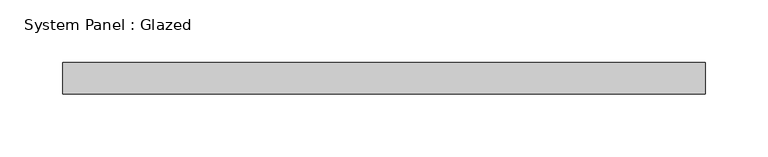
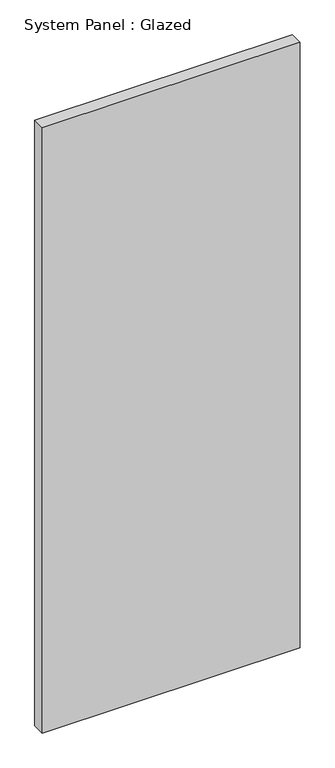
"""IFC4 building model written with IfcOpenShell, lengths in millimetres: plate geometry, System Panel : Glazed."""

from ifc_helpers import new_model, si_unit, origin, origin_with_axes, place, context, project, spatial, polyline, outline, extrude, source, transform, mapped, element, save


def system_panel_glazed_2596f6b1(model_context):
    return source(origin(), model_context, "Body", "SweptSolid", [
        extrude(outline(polyline([(257.175, 19.05), (-257.175, 19.05), (-257.175, 44.45), (257.175, 44.45), (257.175, 19.05)])), origin_with_axes(), (0.0, 0.0, 1.0), 1276.35),
    ])


if __name__ == "__main__":
    model = new_model("IFC4")
    model_context = context("Model", 3, world=origin())
    ifc_project = project(units=[si_unit("LENGTHUNIT", "METRE", prefix="MILLI")], contexts=[model_context])
    site = spatial("IfcSite", under=ifc_project)
    building = spatial("IfcBuilding", under=site)
    placement = place(None, origin())
    system_panel_glazed_shape = system_panel_glazed_2596f6b1(model_context)
    element("IfcPlate", 1, ObjectType="System Panel : Glazed", at=placement, inside=building, context=model_context, shape_type="MappedRepresentation", body=[
        mapped(system_panel_glazed_shape, transform((0.0, 0.0, 0.0), x_axis=(1.0, 0.0, 0.0), y_axis=(0.0, 1.0, 0.0), z_axis=(0.0, 0.0, 1.0))),
    ])
    save(model, "model.ifc")

# Revit data of these elements
# Type "System Panel : Glazed"
#   Construction Type Id = "GSP4R"
#   Analytic Construction = "1/8 in Pilkington single glazing"
#   Visual Light Transmittance = 0.9
#   Solar Heat Gain Coefficient = 0.86
#   Heat Transfer Coefficient (U) = 1.18115 BTU/(h·ft²·°F)
#   Define Thermal Properties by = 1
# Element 1 (IfcPlate, "System Panel : Glazed")
#   Materials on its faces: "Glass"
# Materials
#   "Glass": class "Glass", colour RGB 0 128 192, transparency 0.75, Description = "Soda Lime Glass", Cost = 0
